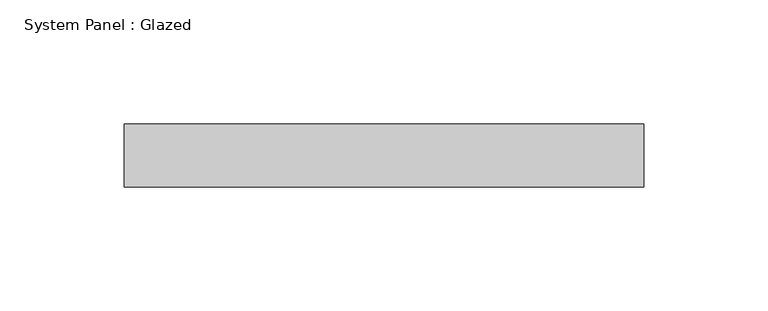
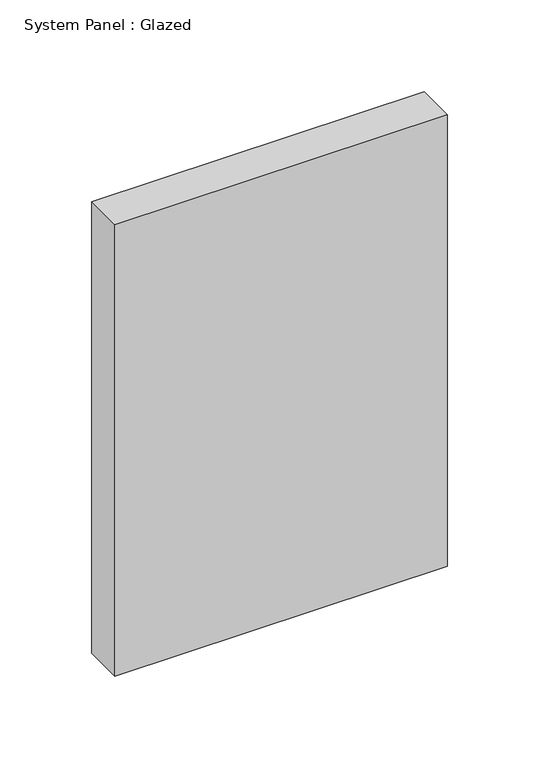
"""IFC4 building model written with IfcOpenShell, lengths in millimetres: plate geometry, System Panel : Glazed."""

from ifc_helpers import new_model, si_unit, origin, origin_with_axes, place, context, project, spatial, polyline, outline, extrude, source, transform, mapped, element, save


def system_panel_glazed_058753b2(model_context):
    return source(origin(), model_context, "Body", "SweptSolid", [
        extrude(outline(polyline([(104.775, 19.05), (-104.775, 19.05), (-104.775, 44.45), (104.775, 44.45), (104.775, 19.05)])), origin_with_axes(), (0.0, 0.0, 1.0), 300.99),
    ])


if __name__ == "__main__":
    model = new_model("IFC4")
    model_context = context("Model", 3, world=origin())
    ifc_project = project(units=[si_unit("LENGTHUNIT", "METRE", prefix="MILLI")], contexts=[model_context])
    site = spatial("IfcSite", under=ifc_project)
    building = spatial("IfcBuilding", under=site)
    placement = place(None, origin())
    system_panel_glazed_shape = system_panel_glazed_058753b2(model_context)
    element("IfcPlate", 1, ObjectType="System Panel : Glazed", at=placement, inside=building, context=model_context, shape_type="MappedRepresentation", body=[
        mapped(system_panel_glazed_shape, transform((0.0, 0.0, 0.0), x_axis=(1.0, 0.0, 0.0), y_axis=(0.0, 1.0, 0.0), z_axis=(0.0, 0.0, 1.0))),
    ])
    save(model, "model.ifc")

# Revit data of these elements
# Type "System Panel : Glazed"
#   Construction Type Id = "GSP4R"
#   Analytic Construction = "1/8 in Pilkington single glazing"
#   Visual Light Transmittance = 0.9
#   Solar Heat Gain Coefficient = 0.86
#   Heat Transfer Coefficient (U) = 1.18115 BTU/(h·ft²·°F)
#   Define Thermal Properties by = 1
# Element 1 (IfcPlate, "System Panel : Glazed")
#   Materials on its faces: "Glass"
# Materials
#   "Glass": class "Glass", colour RGB 0 128 192, transparency 0.75, Description = "Soda Lime Glass", Cost = 0
